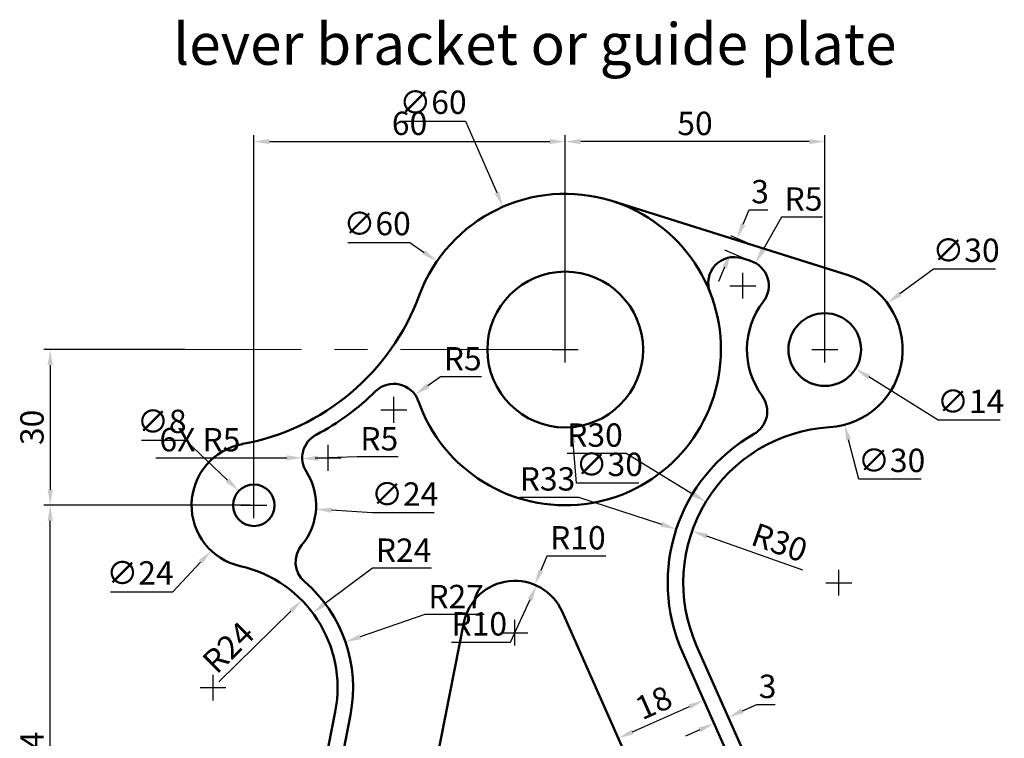
# Model space of a CAD drawing. Units: millimetres. Extents: x 43 to 233, y 2 to 211.
# Tile 2 of 2: x 43 to 233, y 72 to 211. Entities that reach past the tile are written whole.
import ezdxf

# ---------------------------------------------------------------- set-up
doc = ezdxf.new("R2010")
doc.units = ezdxf.units.MM
doc.linetypes.add('CENTER', pattern=[50.8, 31.75, -6.35, 6.35, -6.35])
for name, color, linetype, lineweight in [('M-CNTR', 4, 'CENTER', 18), ('M-DIMS', 2, 'Continuous', 25), ('M-OUTL', 7, 'Continuous', 50), ('M-TEXT', 7, 'Continuous', 25)]:
    doc.layers.add(name, color=color, linetype=linetype, lineweight=lineweight)
doc.styles.get("Standard").update_dxf_attribs({"font": 'arial.ttf'})
doc.dimstyles.new('ISO-25', dxfattribs={"dimtxt": 4.5, "dimasz": 3, "dimexe": 1.25, "dimexo": 0.625, "dimtad": 1, "dimtoh": 1, "dimdec": 0, "dimtxsty": 'Standard', "dimcen": 2.5, "dimadec": 0, "dimazin": 0, "dimtfac": 1, "dimtdec": 0, "dimtofl": 0, "dimtmove": 0, "dimatfit": 3, "dimfxl": 1, "dimarcsym": 0})

# ---------------------------------------------------------------- blocks, each defined once
blk = doc.blocks.new('*D5')
at = {"layer": 'Defpoints', "color": 0, "transparency": 16777216}
for p in [(147.97, 187.22), (147.97, 147.16), (87.97, 117.16)]:
    blk.add_point(p, dxfattribs=at)
at = {"layer": 'M-DIMS', "color": 0, "lineweight": -2, "transparency": 16777216}
for p, q in [((87.97, 117.79), (87.97, 188.47)), ((147.97, 147.79), (147.97, 188.47)), ((90.97, 187.22), (144.97, 187.22))]:
    blk.add_line(p, q, dxfattribs=at)
at = {"layer": 'M-DIMS', "color": 0, "transparency": 16777216}
for points in [[(90.97, 187.72), (90.97, 186.72), (87.97, 187.22)], [(144.97, 187.72), (144.97, 186.72), (147.97, 187.22)]]:
    blk.add_solid(points, dxfattribs=at)
at = {"layer": 'M-DIMS', "color": 0, "transparency": 16777216, "insert": (117.97, 190.15), "char_height": 4.5, "attachment_point": 5}
blk.add_mtext('60', dxfattribs=at)
blk = doc.blocks.new('*D6')
at = {"layer": 'Defpoints', "color": 0, "transparency": 16777216}
for p in [(147.97, 187.21), (147.97, 147.16), (197.97, 147.16)]:
    blk.add_point(p, dxfattribs=at)
at = {"layer": 'M-DIMS', "color": 0, "lineweight": -2, "transparency": 16777216}
for p, q in [((147.97, 147.79), (147.97, 188.46)), ((197.97, 147.79), (197.97, 188.46)), ((194.97, 187.21), (150.97, 187.21))]:
    blk.add_line(p, q, dxfattribs=at)
at = {"layer": 'M-DIMS', "color": 0, "transparency": 16777216}
for points in [[(150.97, 187.71), (150.97, 186.71), (147.97, 187.21)], [(194.97, 187.71), (194.97, 186.71), (197.97, 187.21)]]:
    blk.add_solid(points, dxfattribs=at)
at = {"layer": 'M-DIMS', "color": 0, "transparency": 16777216, "insert": (172.97, 190.13), "char_height": 4.5, "attachment_point": 5}
blk.add_mtext('50', dxfattribs=at)
blk = doc.blocks.new('*D7')
at = {"layer": 'Defpoints', "color": 0, "transparency": 16777216}
for p in [(48.73, 117.16), (87.97, 117.16), (75.97, 23.16)]:
    blk.add_point(p, dxfattribs=at)
at = {"layer": 'M-DIMS', "color": 0, "lineweight": -2, "transparency": 16777216}
for p, q in [((87.34, 117.16), (47.48, 117.16)), ((48.73, 26.16), (48.73, 114.16)), ((75.34, 23.16), (47.48, 23.16))]:
    blk.add_line(p, q, dxfattribs=at)
at = {"layer": 'M-DIMS', "color": 0, "transparency": 16777216}
for points in [[(48.23, 114.16), (49.23, 114.16), (48.73, 117.16)], [(48.23, 26.16), (49.23, 26.16), (48.73, 23.16)]]:
    blk.add_solid(points, dxfattribs=at)
at = {"layer": 'M-DIMS', "color": 0, "transparency": 16777216, "insert": (45.81, 70.16), "char_height": 4.5, "attachment_point": 5, "rotation": 90}
blk.add_mtext('94', dxfattribs=at)
blk = doc.blocks.new('*D8')
at = {"layer": 'Defpoints', "color": 0, "transparency": 16777216}
for p in [(75.36, 147.16), (48.73, 117.16), (64.71, 117.16)]:
    blk.add_point(p, dxfattribs=at)
at = {"layer": 'M-DIMS', "color": 0, "lineweight": -2, "transparency": 16777216}
for p, q in [((74.74, 147.16), (47.48, 147.16)), ((48.73, 144.16), (48.73, 120.16)), ((64.08, 117.16), (47.48, 117.16))]:
    blk.add_line(p, q, dxfattribs=at)
at = {"layer": 'M-DIMS', "color": 0, "transparency": 16777216}
for points in [[(48.23, 144.16), (49.23, 144.16), (48.73, 147.16)], [(48.23, 120.16), (49.23, 120.16), (48.73, 117.16)]]:
    blk.add_solid(points, dxfattribs=at)
at = {"layer": 'M-DIMS', "color": 0, "transparency": 16777216, "insert": (45.8, 132.16), "char_height": 4.5, "attachment_point": 5, "rotation": 90}
blk.add_mtext('30', dxfattribs=at)
blk = doc.blocks.new('*D11')
at = {"layer": 'Defpoints', "color": 0, "transparency": 16777216}
for p in [(123.26, 164.18), (172.67, 130.14)]:
    blk.add_point(p, dxfattribs=at)
at = {"layer": 'M-DIMS', "color": 0, "lineweight": -2, "transparency": 16777216}
for p, q in [((106.06, 167.8), (118.01, 167.8)), ((118.01, 167.8), (120.79, 165.88)), ((147.97, 144.66), (147.97, 149.66)), ((145.47, 147.16), (150.47, 147.16))]:
    blk.add_line(p, q, dxfattribs=at)
at = {"layer": 'M-DIMS', "color": 0, "transparency": 16777216}
blk.add_solid([(121.07, 166.3), (120.51, 165.47), (123.26, 164.18)], dxfattribs=at)
at = {"layer": 'M-DIMS', "color": 0, "transparency": 16777216, "insert": (111.73, 170.84), "char_height": 4.5, "attachment_point": 5}
blk.add_mtext('∅60', dxfattribs=at)
blk = doc.blocks.new('*D12')
at = {"layer": 'Defpoints', "color": 0, "transparency": 16777216}
for p in [(146.69, 162.11), (149.24, 132.22)]:
    blk.add_point(p, dxfattribs=at)
at = {"layer": 'M-DIMS', "color": 0, "lineweight": -2, "transparency": 16777216}
for p, q in [((147.97, 144.66), (147.97, 149.66)), ((145.47, 147.16), (150.47, 147.16)), ((150.17, 121.41), (149.5, 129.23)), ((162.12, 121.41), (150.17, 121.41))]:
    blk.add_line(p, q, dxfattribs=at)
at = {"layer": 'M-DIMS', "color": 0, "transparency": 16777216}
blk.add_solid([(150, 129.27), (149, 129.18), (149.24, 132.22)], dxfattribs=at)
at = {"layer": 'M-DIMS', "color": 0, "transparency": 16777216, "insert": (156.46, 124.46), "char_height": 4.5, "attachment_point": 5}
blk.add_mtext('∅30', dxfattribs=at)
blk = doc.blocks.new('*D13')
at = {"layer": 'Defpoints', "color": 0, "transparency": 16777216}
for p in [(96.18, 125.91), (79.75, 108.41)]:
    blk.add_point(p, dxfattribs=at)
at = {"layer": 'M-DIMS', "color": 0, "lineweight": -2, "transparency": 16777216}
for p, q in [((87.97, 114.66), (87.97, 119.66)), ((85.47, 117.16), (90.47, 117.16)), ((72.33, 100.5), (77.7, 106.22)), ((60.38, 100.5), (72.33, 100.5))]:
    blk.add_line(p, q, dxfattribs=at)
at = {"layer": 'M-DIMS', "color": 0, "transparency": 16777216}
blk.add_solid([(77.34, 106.57), (78.07, 105.88), (79.75, 108.41)], dxfattribs=at)
at = {"layer": 'M-DIMS', "color": 0, "transparency": 16777216, "insert": (66.04, 103.55), "char_height": 4.5, "attachment_point": 5}
blk.add_mtext('∅24', dxfattribs=at)
blk = doc.blocks.new('*D14')
at = {"layer": 'Defpoints', "color": 0, "transparency": 16777216}
for p in [(97.3, 126.15), (102.3, 126.3)]:
    blk.add_point(p, dxfattribs=at)
at = {"layer": 'M-DIMS', "color": 0, "lineweight": -2, "transparency": 16777216}
for p, q in [((107.87, 126.48), (100.3, 126.24)), ((115.79, 126.48), (107.87, 126.48))]:
    blk.add_line(p, q, dxfattribs=at)
at = {"layer": 'M-DIMS', "color": 0, "transparency": 16777216}
blk.add_solid([(100.28, 126.74), (100.31, 125.74), (97.3, 126.15)], dxfattribs=at)
at = {"layer": 'M-DIMS', "color": 0, "transparency": 16777216, "insert": (112.14, 129.39), "char_height": 4.5, "attachment_point": 5}
blk.add_mtext('R5', dxfattribs=at)
blk = doc.blocks.new('*D15')
at = {"layer": 'Defpoints', "color": 0, "transparency": 16777216}
for p in [(97.2, 98.87), (80.1, 82.03)]:
    blk.add_point(p, dxfattribs=at)
at = {"layer": 'M-DIMS', "color": 0, "lineweight": -2, "transparency": 16777216}
blk.add_line((81.2, 83.12), (95.07, 96.76), dxfattribs=at)
at = {"layer": 'M-DIMS', "color": 0, "transparency": 16777216}
blk.add_solid([(94.71, 97.12), (95.42, 96.41), (97.2, 98.87)], dxfattribs=at)
at = {"layer": 'M-DIMS', "color": 0, "transparency": 16777216, "insert": (83.45, 89.38), "char_height": 4.5, "attachment_point": 5, "rotation": 44.5495}
blk.add_mtext('R24', dxfattribs=at)
blk = doc.blocks.new('*D17')
at = {"layer": 'Defpoints', "color": 0, "transparency": 16777216}
for p in [(184.64, 163.82), (182.19, 159.46)]:
    blk.add_point(p, dxfattribs=at)
at = {"layer": 'M-DIMS', "color": 0, "lineweight": -2, "transparency": 16777216}
for p, q in [((189.61, 172.66), (186.11, 166.43)), ((197.53, 172.66), (189.61, 172.66)), ((182.19, 156.96), (182.19, 161.96)), ((179.69, 159.46), (184.69, 159.46))]:
    blk.add_line(p, q, dxfattribs=at)
at = {"layer": 'M-DIMS', "color": 0, "transparency": 16777216}
blk.add_solid([(185.68, 166.68), (186.55, 166.19), (184.64, 163.82)], dxfattribs=at)
at = {"layer": 'M-DIMS', "color": 0, "transparency": 16777216, "insert": (193.88, 175.58), "char_height": 4.5, "attachment_point": 5}
blk.add_mtext('R5', dxfattribs=at)
blk = doc.blocks.new('*D18')
at = {"layer": 'Defpoints', "color": 0, "transparency": 16777216}
for p in [(181.05, 168.55), (184.05, 167.26), (182.86, 164.49)]:
    blk.add_point(p, dxfattribs=at)
at = {"layer": 'M-DIMS', "color": 0, "lineweight": -2, "transparency": 16777216}
for p, q in [((182.23, 171.3), (183.41, 174.06)), ((183.41, 174.06), (186.98, 174.06)), ((183.48, 167.51), (179.9, 169.04)), ((182.29, 164.74), (178.71, 166.27)), ((178.68, 163.02), (177.5, 160.26))]:
    blk.add_line(p, q, dxfattribs=at)
at = {"layer": 'M-DIMS', "color": 0, "transparency": 16777216}
for points in [[(181.77, 171.5), (182.69, 171.11), (181.05, 168.55)], [(178.22, 163.21), (179.14, 162.82), (179.86, 165.77)]]:
    blk.add_solid(points, dxfattribs=at)
at = {"layer": 'M-DIMS', "color": 0, "transparency": 16777216, "insert": (185.51, 176.99), "char_height": 4.5, "attachment_point": 5}
blk.add_mtext('3', dxfattribs=at)
blk = doc.blocks.new('*D19')
at = {"layer": 'Defpoints', "color": 0, "transparency": 16777216}
for p in [(119.03, 138.45), (114.94, 135.57)]:
    blk.add_point(p, dxfattribs=at)
at = {"layer": 'M-DIMS', "color": 0, "lineweight": -2, "transparency": 16777216}
for p, q in [((123.94, 141.9), (121.48, 140.17)), ((131.85, 141.9), (123.94, 141.9)), ((114.94, 133.07), (114.94, 138.07)), ((112.44, 135.57), (117.44, 135.57))]:
    blk.add_line(p, q, dxfattribs=at)
at = {"layer": 'M-DIMS', "color": 0, "transparency": 16777216}
blk.add_solid([(121.2, 140.58), (121.77, 139.77), (119.03, 138.45)], dxfattribs=at)
at = {"layer": 'M-DIMS', "color": 0, "transparency": 16777216, "insert": (128.21, 144.82), "char_height": 4.5, "attachment_point": 5}
blk.add_mtext('R5', dxfattribs=at)
blk = doc.blocks.new('*D20')
at = {"layer": 'Defpoints', "color": 0, "transparency": 16777216}
for p in [(142.44, 101.7), (138.24, 92.62)]:
    blk.add_point(p, dxfattribs=at)
at = {"layer": 'M-DIMS', "color": 0, "lineweight": -2, "transparency": 16777216}
for p, q in [((137.41, 90.81), (141.18, 98.98)), ((126.04, 90.81), (137.41, 90.81))]:
    blk.add_line(p, q, dxfattribs=at)
at = {"layer": 'M-DIMS', "color": 0, "transparency": 16777216}
blk.add_solid([(140.73, 99.19), (141.63, 98.77), (142.44, 101.7)], dxfattribs=at)
at = {"layer": 'M-DIMS', "color": 0, "transparency": 16777216, "insert": (131.41, 93.74), "char_height": 4.5, "attachment_point": 5}
blk.add_mtext('R10', dxfattribs=at)
blk = doc.blocks.new('*D24')
at = {"layer": 'Defpoints', "color": 0, "transparency": 16777216}
for p in [(174.65, 79.59), (179.84, 67.89), (163.39, 60.6)]:
    blk.add_point(p, dxfattribs=at)
at = {"layer": 'M-DIMS', "color": 0, "lineweight": -2, "transparency": 16777216}
for p, q in [((179.59, 68.46), (174.15, 80.74)), ((160.94, 73.51), (171.91, 78.38)), ((163.14, 61.17), (157.69, 73.44))]:
    blk.add_line(p, q, dxfattribs=at)
at = {"layer": 'M-DIMS', "color": 0, "transparency": 16777216}
for points in [[(171.71, 78.83), (172.11, 77.92), (174.65, 79.59)], [(160.74, 73.97), (161.15, 73.05), (158.2, 72.29)]]:
    blk.add_solid(points, dxfattribs=at)
at = {"layer": 'M-DIMS', "color": 0, "transparency": 16777216, "insert": (165.24, 78.62), "char_height": 4.5, "attachment_point": 5, "rotation": 23.9196}
blk.add_mtext('18', dxfattribs=at)
blk = doc.blocks.new('*D25')
at = {"layer": 'Defpoints', "color": 0, "transparency": 16777216}
for p in [(179.38, 76.34), (176.87, 74.6), (179.61, 75.82)]:
    blk.add_point(p, dxfattribs=at)
at = {"layer": 'M-DIMS', "color": 0, "lineweight": -2, "transparency": 16777216}
for p, q in [((182.12, 77.56), (184.86, 78.77)), ((184.86, 78.77), (188.43, 78.77)), ((176.62, 75.17), (176.13, 76.27)), ((179.36, 76.39), (178.87, 77.48)), ((173.89, 73.91), (171.15, 72.69))]:
    blk.add_line(p, q, dxfattribs=at)
at = {"layer": 'M-DIMS', "color": 0, "transparency": 16777216}
for points in [[(181.92, 78.02), (182.32, 77.1), (179.38, 76.34)], [(173.69, 74.37), (174.1, 73.45), (176.64, 75.13)]]:
    blk.add_solid(points, dxfattribs=at)
at = {"layer": 'M-DIMS', "color": 0, "transparency": 16777216, "insert": (186.96, 81.7), "char_height": 4.5, "attachment_point": 5}
blk.add_mtext('3', dxfattribs=at)
blk = doc.blocks.new('*D26')
at = {"layer": 'Defpoints', "color": 0, "transparency": 16777216}
for p in [(85.07, 119.92), (90.87, 114.41)]:
    blk.add_point(p, dxfattribs=at)
at = {"layer": 'M-DIMS', "color": 0, "lineweight": -2, "transparency": 16777216}
for p, q in [((66.31, 129.69), (74.79, 129.69)), ((74.79, 129.69), (82.89, 121.98)), ((87.97, 114.66), (87.97, 119.66)), ((85.47, 117.16), (90.47, 117.16))]:
    blk.add_line(p, q, dxfattribs=at)
at = {"layer": 'M-DIMS', "color": 0, "transparency": 16777216}
blk.add_solid([(83.24, 122.35), (82.55, 121.62), (85.07, 119.92)], dxfattribs=at)
at = {"layer": 'M-DIMS', "color": 0, "transparency": 16777216, "insert": (70.23, 132.74), "char_height": 4.5, "attachment_point": 5}
blk.add_mtext('∅8', dxfattribs=at)
blk = doc.blocks.new('*D27')
at = {"layer": 'Defpoints', "color": 0, "transparency": 16777216}
for p in [(172.41, 112.2), (200.71, 102.25)]:
    blk.add_point(p, dxfattribs=at)
at = {"layer": 'M-DIMS', "color": 0, "lineweight": -2, "transparency": 16777216}
blk.add_line((193.76, 104.69), (175.24, 111.2), dxfattribs=at)
at = {"layer": 'M-DIMS', "color": 0, "transparency": 16777216}
blk.add_solid([(175.4, 111.67), (175.07, 110.73), (172.41, 112.2)], dxfattribs=at)
at = {"layer": 'M-DIMS', "color": 0, "transparency": 16777216, "insert": (189.07, 109.44), "char_height": 4.5, "attachment_point": 5, "rotation": 340.6292}
blk.add_mtext('R30', dxfattribs=at)
blk = doc.blocks.new('*D28')
at = {"layer": 'Defpoints', "color": 0, "transparency": 16777216}
for p in [(210.03, 156.08), (185.91, 138.24)]:
    blk.add_point(p, dxfattribs=at)
at = {"layer": 'M-DIMS', "color": 0, "lineweight": -2, "transparency": 16777216}
for p, q in [((218.92, 162.65), (212.44, 157.86)), ((230.87, 162.65), (218.92, 162.65)), ((197.97, 144.66), (197.97, 149.66)), ((195.47, 147.16), (200.47, 147.16))]:
    blk.add_line(p, q, dxfattribs=at)
at = {"layer": 'M-DIMS', "color": 0, "transparency": 16777216}
blk.add_solid([(212.14, 158.27), (212.74, 157.46), (210.03, 156.08)], dxfattribs=at)
at = {"layer": 'M-DIMS', "color": 0, "transparency": 16777216, "insert": (225.2, 165.7), "char_height": 4.5, "attachment_point": 5}
blk.add_mtext('∅30', dxfattribs=at)
blk = doc.blocks.new('*D29')
at = {"layer": 'Defpoints', "color": 0, "transparency": 16777216}
for p in [(192.03, 150.87), (203.91, 143.46)]:
    blk.add_point(p, dxfattribs=at)
at = {"layer": 'M-DIMS', "color": 0, "lineweight": -2, "transparency": 16777216}
for p, q in [((197.97, 144.66), (197.97, 149.66)), ((195.47, 147.16), (200.47, 147.16)), ((219.81, 133.54), (206.45, 141.87)), ((231.75, 133.54), (219.81, 133.54))]:
    blk.add_line(p, q, dxfattribs=at)
at = {"layer": 'M-DIMS', "color": 0, "transparency": 16777216}
blk.add_solid([(206.72, 142.29), (206.19, 141.45), (203.91, 143.46)], dxfattribs=at)
at = {"layer": 'M-DIMS', "color": 0, "transparency": 16777216, "insert": (226.09, 136.59), "char_height": 4.5, "attachment_point": 5}
blk.add_mtext('∅14', dxfattribs=at)
blk = doc.blocks.new('*D32')
at = {"layer": 'Defpoints', "color": 0, "transparency": 16777216}
for p in [(135.97, 174.66), (159.96, 119.66)]:
    blk.add_point(p, dxfattribs=at)
at = {"layer": 'M-DIMS', "color": 0, "lineweight": -2, "transparency": 16777216}
for p, q in [((116.83, 191.16), (128.78, 191.16)), ((128.78, 191.16), (134.77, 177.41)), ((147.97, 144.66), (147.97, 149.66)), ((145.47, 147.16), (150.47, 147.16))]:
    blk.add_line(p, q, dxfattribs=at)
at = {"layer": 'M-DIMS', "color": 0, "transparency": 16777216}
blk.add_solid([(135.23, 177.61), (134.32, 177.21), (135.97, 174.66)], dxfattribs=at)
at = {"layer": 'M-DIMS', "color": 0, "transparency": 16777216, "insert": (122.49, 194.21), "char_height": 4.5, "attachment_point": 5}
blk.add_mtext('∅60', dxfattribs=at)
blk = doc.blocks.new('*D33')
at = {"layer": 'Defpoints', "color": 0, "transparency": 16777216}
for p in [(175.07, 117.83), (200.71, 102.25)]:
    blk.add_point(p, dxfattribs=at)
at = {"layer": 'M-DIMS', "color": 0, "lineweight": -2, "transparency": 16777216}
for p, q in [((148.33, 127.18), (159.69, 127.18)), ((159.69, 127.18), (172.51, 119.39)), ((200.71, 99.75), (200.71, 104.75)), ((198.21, 102.25), (203.21, 102.25))]:
    blk.add_line(p, q, dxfattribs=at)
at = {"layer": 'M-DIMS', "color": 0, "transparency": 16777216}
blk.add_solid([(172.77, 119.81), (172.25, 118.96), (175.07, 117.83)], dxfattribs=at)
at = {"layer": 'M-DIMS', "color": 0, "transparency": 16777216, "insert": (153.7, 130.1), "char_height": 4.5, "attachment_point": 5}
blk.add_mtext('R30', dxfattribs=at)
blk = doc.blocks.new('*D34')
at = {"layer": 'Defpoints', "color": 0, "transparency": 16777216}
for p in [(194.13, 161.66), (201.8, 132.66)]:
    blk.add_point(p, dxfattribs=at)
at = {"layer": 'M-DIMS', "color": 0, "lineweight": -2, "transparency": 16777216}
for p, q in [((197.97, 144.66), (197.97, 149.66)), ((195.47, 147.16), (200.47, 147.16)), ((204.57, 122.17), (202.57, 129.76)), ((216.52, 122.17), (204.57, 122.17))]:
    blk.add_line(p, q, dxfattribs=at)
at = {"layer": 'M-DIMS', "color": 0, "transparency": 16777216}
blk.add_solid([(203.05, 129.89), (202.08, 129.63), (201.8, 132.66)], dxfattribs=at)
at = {"layer": 'M-DIMS', "color": 0, "transparency": 16777216, "insert": (210.86, 125.22), "char_height": 4.5, "attachment_point": 5}
blk.add_mtext('∅30', dxfattribs=at)
blk = doc.blocks.new('*D35')
at = {"layer": 'Defpoints', "color": 0, "transparency": 16777216}
for p in [(75.99, 117.93), (99.94, 116.39)]:
    blk.add_point(p, dxfattribs=at)
at = {"layer": 'M-DIMS', "color": 0, "lineweight": -2, "transparency": 16777216}
for p, q in [((87.97, 114.66), (87.97, 119.66)), ((85.47, 117.16), (90.47, 117.16)), ((110.77, 115.69), (102.94, 116.2)), ((122.71, 115.69), (110.77, 115.69))]:
    blk.add_line(p, q, dxfattribs=at)
at = {"layer": 'M-DIMS', "color": 0, "transparency": 16777216}
blk.add_solid([(102.97, 116.7), (102.9, 115.7), (99.94, 116.39)], dxfattribs=at)
at = {"layer": 'M-DIMS', "color": 0, "transparency": 16777216, "insert": (117.05, 118.74), "char_height": 4.5, "attachment_point": 5}
blk.add_mtext('∅24', dxfattribs=at)
blk = doc.blocks.new('*D36')
at = {"layer": 'Defpoints', "color": 0, "transparency": 16777216}
for p in [(97.3, 126.3), (102.3, 126.3)]:
    blk.add_point(p, dxfattribs=at)
at = {"layer": 'M-DIMS', "color": 0, "lineweight": -2, "transparency": 16777216}
for p, q in [((102.3, 123.8), (102.3, 128.8)), ((69.09, 126.29), (86.7, 126.29)), ((86.7, 126.29), (94.3, 126.3)), ((99.8, 126.3), (104.8, 126.3))]:
    blk.add_line(p, q, dxfattribs=at)
at = {"layer": 'M-DIMS', "color": 0, "transparency": 16777216}
blk.add_solid([(94.3, 126.8), (94.3, 125.8), (97.3, 126.3)], dxfattribs=at)
at = {"layer": 'M-DIMS', "color": 0, "transparency": 16777216, "insert": (77.59, 129.21), "char_height": 4.5, "attachment_point": 5}
blk.add_mtext('6X R5', dxfattribs=at)
blk = doc.blocks.new('*D37')
at = {"layer": 'Defpoints', "color": 0, "transparency": 16777216}
for p in [(169.36, 112.55), (200.71, 102.25)]:
    blk.add_point(p, dxfattribs=at)
at = {"layer": 'M-DIMS', "color": 0, "lineweight": -2, "transparency": 16777216}
for p, q in [((139.17, 118.74), (150.55, 118.74)), ((150.55, 118.74), (166.51, 113.49)), ((200.71, 99.75), (200.71, 104.75)), ((198.21, 102.25), (203.21, 102.25))]:
    blk.add_line(p, q, dxfattribs=at)
at = {"layer": 'M-DIMS', "color": 0, "transparency": 16777216}
blk.add_solid([(166.66, 113.96), (166.35, 113.01), (169.36, 112.55)], dxfattribs=at)
at = {"layer": 'M-DIMS', "color": 0, "transparency": 16777216, "insert": (144.55, 121.66), "char_height": 4.5, "attachment_point": 5}
blk.add_mtext('R33', dxfattribs=at)
blk = doc.blocks.new('*D38')
at = {"layer": 'Defpoints', "color": 0, "transparency": 16777216}
for p in [(105.62, 90.84), (80.1, 82.03)]:
    blk.add_point(p, dxfattribs=at)
at = {"layer": 'M-DIMS', "color": 0, "lineweight": -2, "transparency": 16777216}
for p, q in [((120.94, 96.12), (108.46, 91.81)), ((132.32, 96.12), (120.94, 96.12)), ((80.1, 79.53), (80.1, 84.53)), ((77.6, 82.03), (82.6, 82.03))]:
    blk.add_line(p, q, dxfattribs=at)
at = {"layer": 'M-DIMS', "color": 0, "transparency": 16777216}
blk.add_solid([(108.3, 92.29), (108.62, 91.34), (105.62, 90.84)], dxfattribs=at)
at = {"layer": 'M-DIMS', "color": 0, "transparency": 16777216, "insert": (126.94, 99), "char_height": 4.5, "attachment_point": 5}
blk.add_mtext('R27', dxfattribs=at)
blk = doc.blocks.new('*D39')
at = {"layer": 'Defpoints', "color": 0, "transparency": 16777216}
for p in [(99.31, 96.42), (80.1, 82.03)]:
    blk.add_point(p, dxfattribs=at)
at = {"layer": 'M-DIMS', "color": 0, "lineweight": -2, "transparency": 16777216}
for p, q in [((110.84, 105.05), (101.71, 98.22)), ((122.2, 105.05), (110.84, 105.05)), ((80.1, 79.53), (80.1, 84.53)), ((77.6, 82.03), (82.6, 82.03))]:
    blk.add_line(p, q, dxfattribs=at)
at = {"layer": 'M-DIMS', "color": 0, "transparency": 16777216}
blk.add_solid([(101.41, 98.62), (102.01, 97.82), (99.31, 96.42)], dxfattribs=at)
at = {"layer": 'M-DIMS', "color": 0, "transparency": 16777216, "insert": (116.83, 107.93), "char_height": 4.5, "attachment_point": 5}
blk.add_mtext('R24', dxfattribs=at)
blk = doc.blocks.new('*D40')
at = {"layer": 'Defpoints', "color": 0, "transparency": 16777216}
for p in [(142.1, 101.85), (138.24, 92.62)]:
    blk.add_point(p, dxfattribs=at)
at = {"layer": 'M-DIMS', "color": 0, "lineweight": -2, "transparency": 16777216}
for p, q in [((144.41, 107.39), (143.26, 104.62)), ((155.78, 107.39), (144.41, 107.39)), ((138.24, 90.12), (138.24, 95.12)), ((135.74, 92.62), (140.74, 92.62))]:
    blk.add_line(p, q, dxfattribs=at)
at = {"layer": 'M-DIMS', "color": 0, "transparency": 16777216}
blk.add_solid([(142.8, 104.81), (143.72, 104.43), (142.1, 101.85)], dxfattribs=at)
at = {"layer": 'M-DIMS', "color": 0, "transparency": 16777216, "insert": (150.41, 110.31), "char_height": 4.5, "attachment_point": 5}
blk.add_mtext('R10', dxfattribs=at)

msp = doc.modelspace()

# ---------------------------------------------------------------- linework, layer by layer
at = {"layer": 'M-CNTR'}
msp.add_line((147.97, 147.16), (70.7, 147.16), dxfattribs=at)
at = {"layer": 'M-OUTL'}
for p, q in [((156.97, 175.78), (202.47, 161.47)), ((182.03, 164.75), (183.69, 164.23)), ((164.54, 58), (147.38, 96.68)), ((120.94, 56.51), (128.43, 94.56)), ((195.73, 39.49), (173.28, 90.08)), ((180.99, 65.3), (170.54, 88.87)), ((98.04, 48.91), (103.65, 77.39)), ((103.28, 59.99), (106.59, 76.81))]:
    msp.add_line(p, q, dxfattribs=at)
for centre, radius in [((147.97, 147.16), 15), ((197.97, 147.16), 7), ((87.97, 117.16), 4)]:
    msp.add_circle(centre, radius, dxfattribs=at)
for centre, radius, start, end in [((147.97, 147.16), 30, 72.5424, 159.6704), ((147.97, 147.16), 30, 199.3422, 72.5424), ((180.53, 159.98), 5, 72.5424, 201.4872), ((182.19, 159.46), 5, 322.0551, 72.5424), ((197.97, 147.16), 15, 273.4924, 72.5424), ((77.64, 173.22), 45, 280.4395, 339.6704), ((197.97, 147.16), 15, 142.0551, 216.5171), ((114.94, 135.57), 5, 19.3422, 134.7362), ((77.64, 173.22), 48, 297.7288, 314.7362), ((181.89, 135.26), 5, 299.6781, 36.5171), ((200.71, 102.25), 33, 119.6781, 203.9196), ((200.71, 102.25), 30, 93.4924, 203.9196), ((102.3, 126.3), 5, 117.7288, 212.5356), ((87.97, 117.16), 12, 100.4395, 257.3793), ((87.97, 117.16), 12, 320.0997, 32.5356), ((101.01, 106.26), 5, 140.0997, 229.2044), ((80.1, 82.03), 24, 348.8574, 77.3793), ((80.1, 82.03), 27, 348.8574, 49.2044), ((138.24, 92.62), 10, 23.9196, 168.8574)]:
    msp.add_arc(centre, radius, start, end, dxfattribs=at)

# ---------------------------------------------------------------- texts
at = {"layer": 'M-TEXT', "insert": (72.42, 210.01), "char_height": 8, "attachment_point": 1}
msp.add_mtext_dynamic_manual_height_columns('lever bracket or guide plate', width=172.7557, gutter_width=12.5, heights=[0], dxfattribs=at)

# ---------------------------------------------------------------- dimensions: what is measured, and where the dimension line sits
at = {"layer": 'M-DIMS'}
for p1, p2, override, picture, middle in [((159.96, 119.66), (135.97, 174.66), {"dimdec": 0, "dimlfac": 1, "dimrnd": 0, "dimzin": 0, "dimdsep": 46, "dimlunit": 2}, '*D32', (122.49, 191.16)), ((172.67, 130.14), (123.26, 164.18), {"dimclrd": 0, "dimclre": 0, "dimclrt": 0}, '*D11', (111.73, 167.8)), ((185.91, 138.24), (210.03, 156.08), {"dimclrd": 0, "dimclre": 0, "dimclrt": 0}, '*D28', (225.2, 162.65)), ((194.13, 161.66), (201.8, 132.66), {"dimdec": 0, "dimlfac": 1, "dimrnd": 0, "dimzin": 0, "dimdsep": 46, "dimlunit": 2}, '*D34', (210.86, 122.17)), ((192.03, 150.87), (203.91, 143.46), {"dimclrd": 0, "dimclre": 0, "dimclrt": 0}, '*D29', (226.09, 133.54)), ((90.87, 114.41), (85.07, 119.92), {"dimclrd": 0, "dimclre": 0, "dimclrt": 0}, '*D26', (70.23, 129.69))]:
    dim = msp.add_diameter_dim_2p(p1=p1, p2=p2, dimstyle='ISO-25', override=override, dxfattribs=at)
    dim.commit()
    dim.dimension.update_dxf_attribs({"geometry": picture, "text_midpoint": middle, "dimtype": 163})
for base, p1, picture, middle in [((147.97, 187.22), (87.97, 117.16), '*D5', (117.97, 190.15)), ((147.97, 187.21), (197.97, 147.16), '*D6', (172.97, 190.13))]:
    dim = msp.add_linear_dim(base=base, p1=p1, p2=(147.97, 147.16), dimstyle='ISO-25', override={"dimclrd": 0, "dimclre": 0, "dimclrt": 0}, dxfattribs=at)
    dim.commit()
    dim.dimension.update_dxf_attribs({"geometry": picture, "text_midpoint": middle})
for p1, p2, distance, picture, middle in [((182.86, 164.49), (184.05, 167.26), 3.26, '*D18', (185.51, 176.99)), ((176.87, 74.6), (179.61, 75.82), 0.57, '*D25', (186.96, 81.7)), ((163.39, 60.6), (179.84, 67.89), 12.8, '*D24', (165.24, 78.62))]:
    dim = msp.add_aligned_dim(p1=p1, p2=p2, distance=distance, dimstyle='ISO-25', override={"dimclrd": 0, "dimclre": 0, "dimclrt": 0}, dxfattribs=at)
    dim.commit()
    dim.dimension.update_dxf_attribs({"geometry": picture, "text_midpoint": middle})
for center, mpoint, override, picture, middle in [((182.19, 159.46), (184.64, 163.82), {"dimclrd": 0, "dimclre": 0, "dimclrt": 0}, '*D17', (193.88, 172.66)), ((200.71, 102.25), (175.07, 117.83), {"dimdec": 0, "dimlfac": 1, "dimrnd": 0, "dimzin": 0, "dimdsep": 46, "dimlunit": 2}, '*D33', (153.7, 127.18)), ((102.3, 126.3), (97.3, 126.15), {"dimclrd": 0, "dimclre": 0, "dimclrt": 0}, '*D14', (107.87, 126.48)), ((200.71, 102.25), (169.36, 112.55), {"dimdec": 0, "dimlfac": 1, "dimrnd": 0, "dimzin": 0, "dimdsep": 46, "dimlunit": 2}, '*D37', (144.55, 118.74)), ((200.71, 102.25), (172.41, 112.2), {"dimclrd": 0, "dimclre": 0, "dimclrt": 0}, '*D27', (188.1, 106.68)), ((138.24, 92.62), (142.1, 101.85), {"dimdec": 0, "dimlfac": 1, "dimrnd": 0, "dimzin": 0, "dimdsep": 46, "dimlunit": 2}, '*D40', (150.41, 107.39)), ((80.1, 82.03), (99.31, 96.42), {"dimdec": 0, "dimlfac": 1, "dimrnd": 0, "dimzin": 0, "dimdsep": 46, "dimlunit": 2}, '*D39', (116.83, 105.05)), ((80.1, 82.03), (105.62, 90.84), {"dimdec": 0, "dimlfac": 1, "dimrnd": 0, "dimzin": 0, "dimdsep": 46, "dimlunit": 2}, '*D38', (126.94, 96.12)), ((138.24, 92.62), (142.44, 101.7), {"dimclrd": 0, "dimclre": 0, "dimclrt": 0}, '*D20', (131.41, 90.81)), ((80.1, 82.03), (97.2, 98.87), {"dimclrd": 0, "dimclre": 0, "dimclrt": 0}, '*D15', (85.47, 87.32))]:
    dim = msp.add_radius_dim(center=center, mpoint=mpoint, dimstyle='ISO-25', override=override, dxfattribs=at)
    dim.commit()
    dim.dimension.update_dxf_attribs({"geometry": picture, "text_midpoint": middle, "dimtype": 164})
for p1, p2, override, picture, middle in [((146.69, 162.11), (149.24, 132.22), {"dimclrd": 0, "dimclre": 0, "dimclrt": 0}, '*D12', (156.46, 124.46)), ((96.18, 125.91), (79.75, 108.41), {"dimclrd": 0, "dimclre": 0, "dimclrt": 0}, '*D13', (66.04, 103.55)), ((75.99, 117.93), (99.94, 116.39), {"dimdec": 0, "dimlfac": 1, "dimrnd": 0, "dimzin": 0, "dimdsep": 46, "dimlunit": 2}, '*D35', (110.77, 115.69))]:
    dim = msp.add_diameter_dim_2p(p1=p1, p2=p2, dimstyle='ISO-25', override=override, dxfattribs=at)
    dim.commit()
    dim.dimension.update_dxf_attribs({"geometry": picture, "text_midpoint": middle})
for p1, p2, picture, middle in [((75.36, 147.16), (64.71, 117.16), '*D8', (45.8, 132.16)), ((75.97, 23.16), (87.97, 117.16), '*D7', (45.81, 70.16))]:
    dim = msp.add_linear_dim(base=(48.73, 117.16), p1=p1, p2=p2, angle=90, dimstyle='ISO-25', override={"dimclrd": 0, "dimclre": 0, "dimclrt": 0}, dxfattribs=at)
    dim.commit()
    dim.dimension.update_dxf_attribs({"geometry": picture, "text_midpoint": middle})
dim = msp.add_radius_dim(center=(114.94, 135.57), mpoint=(119.03, 138.45), dimstyle='ISO-25', override={"dimclrd": 0, "dimclre": 0, "dimclrt": 0}, dxfattribs=at)
dim.commit()
dim.dimension.update_dxf_attribs({"geometry": '*D19', "text_midpoint": (128.21, 144.82)})
dim = msp.add_radius_dim(center=(102.3, 126.3), mpoint=(97.3, 126.3), text='6X <>', dimstyle='ISO-25', override={"dimdec": 0, "dimlfac": 1, "dimrnd": 0, "dimzin": 0, "dimdsep": 46, "dimlunit": 2}, dxfattribs=at)
dim.commit()
dim.dimension.update_dxf_attribs({"geometry": '*D36', "text_midpoint": (77.59, 129.21)})

doc.saveas('drawing.dxf')
